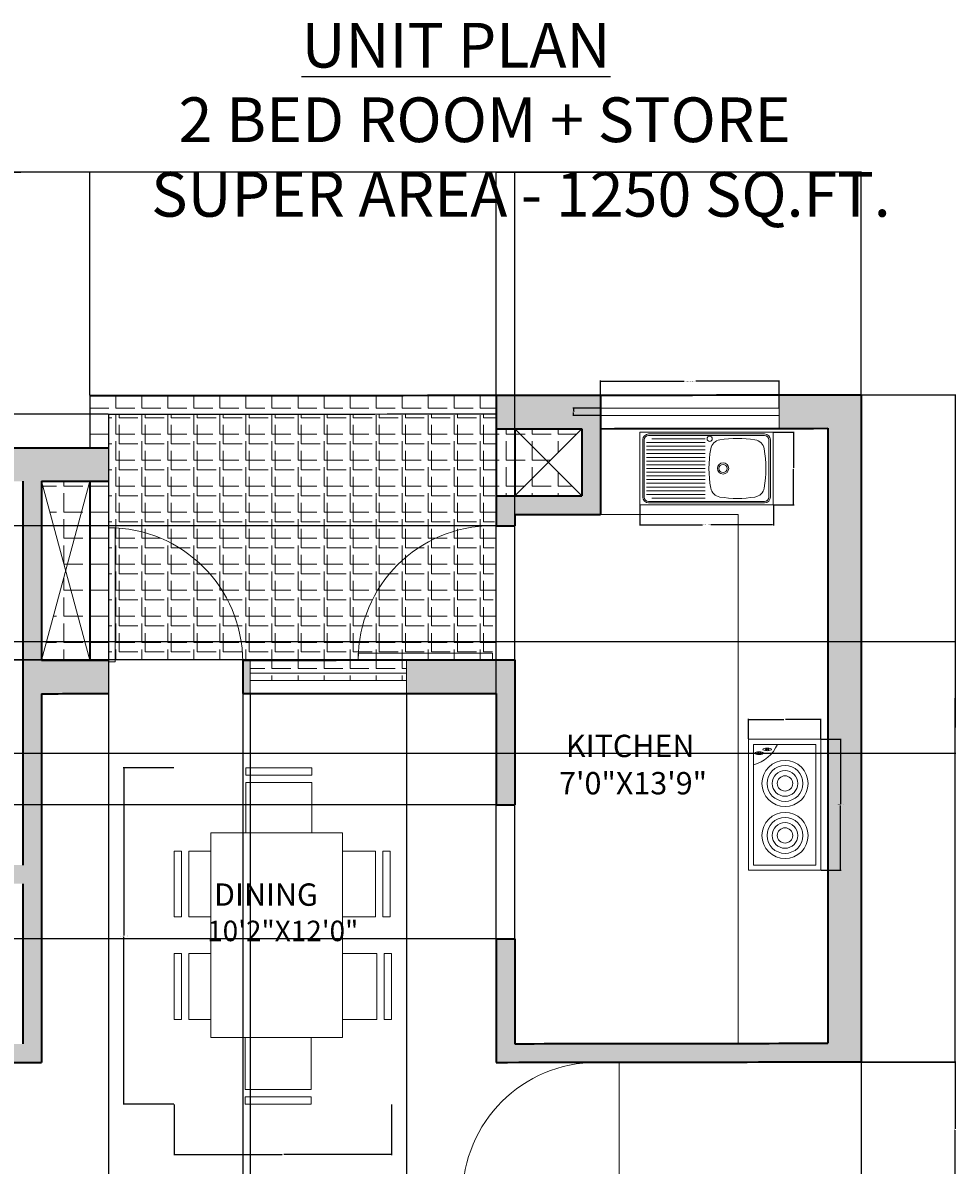
# Model space of a CAD drawing. Units: inches. Extents: x 1044 to 1567, y 918 to 1417.
# Tile 4 of 4: x 1316 to 1567, y 1110 to 1417. Entities that reach past the tile are written whole.
import ezdxf

# ---------------------------------------------------------------- set-up
doc = ezdxf.new("R2010")
doc.units = ezdxf.units.IN
for name, color, linetype, lineweight in [('A-ANNO-DIMS', 2, 'Continuous', 18), ('A-ANNO-TEXT', 7, 'Continuous', 25), ('A-AREA-IDEN', 7, 'Continuous', 18), ('A-EQPM', 8, 'Continuous', 18), ('A-FLOR', 7, 'Continuous', 13), ('A-FLOR-CASE', 8, 'Continuous', 18), ('A-FLOR-FIXT', 9, 'Continuous', 18), ('A-FLOR-OPEN', 8, 'Continuous', 13), ('A-FLOR-PATT', 9, 'Continuous', 13), ('A-FURN', 8, 'Continuous', 18), ('A-GLAZ', 4, 'Continuous', 13), ('A-WALL', 7, 'Continuous', 35), ('A-WALL-PATT', 252, 'Continuous', 13), ('A-WALL-PRPT', 7, 'Continuous', 25), ('door', 4, 'Continuous', 18)]:
    doc.layers.add(name, color=color, linetype=linetype, lineweight=lineweight)
doc.styles.get("Standard").update_dxf_attribs({"font": 'arial.ttf'})
doc.dimstyles.get("Standard").update_dxf_attribs({"dimtxt": 0.18, "dimasz": 0.18, "dimexe": 0.18, "dimexo": 0.0625, "dimgap": 0.09, "dimtad": 0, "dimtih": 1, "dimtoh": 1, "dimdec": 4, "dimzin": 0, "dimdsep": 46, "dimtxsty": 'Standard', "dimcen": 0.09, "dimadec": 0, "dimazin": 0, "dimtfac": 1, "dimtdec": 4, "dimtofl": 0, "dimtmove": 0, "dimatfit": 3, "dimfxl": 1, "dimtolj": 1, "dimtzin": 0, "dimarcsym": 0})

# ---------------------------------------------------------------- blocks, each defined once
blk = doc.blocks.new('*U5')
for p, q in [((-36, 0), (-36, 6)), ((0, 0), (0, 6))]:
    blk.add_line(p, q)
blk.add_lwpolyline([(0, 0), (0, -36), (-1.75, -36), (-1.75, 0)], close=True)
blk.add_arc((0, 0), 36, 180, 270)
blk = doc.blocks.new('*U2')
for p, q in [((0, 0), (0, -6)), ((36, 0), (36, -6))]:
    blk.add_line(p, q)
blk.add_lwpolyline([(0, 0), (0, 36), (1.75, 36), (1.75, 0)], close=True)
blk.add_arc((0, 0), 36, 0, 90)
blk = doc.blocks.new('A$C38705599')
for p, q in [((510, 282), (0, 282)), ((0, 282), (0, 0)), ((510, 0), (510, 282)), ((490, 262), (20, 262)), ((20, 262), (20, 20)), ((490, 20), (490, 262)), ((20, 20), (490, 20)), ((0, 0), (510, 0))]:
    blk.add_line(p, q)
for centre, radius in [((135.4, 139.5), 89.9), ((337.9, 139.5), 89.9), ((455.9, 243.8), 2.39), ((455.9, 235.1), 2.39), ((135.4, 139.5), 69.9), ((135.4, 139.5), 49.9), ((337.9, 139.5), 69.9), ((337.9, 139.5), 49.9), ((470.5, 213.1), 2.39), ((470.5, 204.3), 2.39), ((135.4, 139.5), 29.9), ((337.9, 139.5), 29.9)]:
    blk.add_circle(centre, radius)
blk.add_arc((552.1, 302.1), 147.4, 195.7794, 245.1074)
for centre in [(455.9, 239.9), (470.6, 209.1)]:
    blk.add_ellipse(centre, major_axis=(0, 17), ratio=0.307925)
blk = doc.blocks.new('A$C0C3933DC')
for p, q in [((0, 490), (0, 0)), ((900, 490), (0, 490)), ((59.5, 477.5), (450, 477.5)), ((59.5, 467.5), (450, 467.5)), ((840.5, 477.5), (450, 477.5)), ((840.5, 467.5), (450, 467.5)), ((900, 0), (900, 490)), ((19.5, 52.5), (19.5, 437.5)), ((29.5, 52.5), (29.5, 437.5)), ((441, 420), (45, 420)), ((441, 395), (45, 395)), ((441, 445), (80.7, 445)), ((870.5, 52.5), (870.5, 437.5)), ((880.5, 52.5), (880.5, 437.5)), ((441, 370), (45, 370)), ((441, 345), (45, 345)), ((441, 320), (45, 320)), ((441, 295), (45, 295)), ((441, 270), (45, 270)), ((441, 245), (45, 245)), ((441, 220), (45, 220)), ((441, 195), (45, 195)), ((441, 170), (45, 170)), ((441, 145), (45, 145)), ((441, 120), (45, 120)), ((441, 95), (45, 95)), ((0, 0), (900, 0)), ((441, 70), (45, 70)), ((450, 22.5), (59.5, 22.5)), ((450, 12.5), (59.5, 12.5)), ((441, 45), (80.7, 45)), ((450, 22.5), (840.5, 22.5)), ((450, 12.5), (840.5, 12.5))]:
    blk.add_line(p, q)
for centre, radius in [((471, 445), 17.5), ((561, 245), 38), ((561, 245), 27.5)]:
    blk.add_circle(centre, radius)
for centre, radius, start, end in [((59.5, 437.5), 40, 90, 180), ((59.5, 437.5), 30, 90, 180), ((840.5, 437.5), 40, 0, 90), ((840.5, 437.5), 30, 0, 90), ((551.5, 363.5), 75, 99.07872, 169.88522), ((658, -303), 750, 80.92128, 99.07872), ((764.5, 363.5), 75, 10.11478, 80.92128), ((1216, 245), 750, 169.88522, 190.11478), ((100, 245), 750, 349.88522, 10.11478), ((551.5, 126.5), 75, 190.11478, 260.92128), ((764.5, 126.5), 75, 279.07872, 349.88522), ((59.5, 52.5), 40, 180, 270), ((59.5, 52.5), 30, 180, 270), ((658, 793), 750, 260.92128, 279.07872), ((840.5, 52.5), 30, 270, 0), ((840.5, 52.5), 40, 270, 0)]:
    blk.add_arc(centre, radius, start, end)
blk = doc.blocks.new('A$C6F2E0C66')
for p, q in [((1.2673, 1.4847), (1.2673, 1.4347)), ((1.7173, 1.4847), (1.2673, 1.4847)), ((1.7173, 1.4347), (1.7173, 1.4847)), ((0.5675, 1.4758), (0.5675, 1.4258)), ((1.0175, 1.4758), (0.5675, 1.4758)), ((0.5675, 1.4258), (1.0175, 1.4258)), ((1.0175, 1.4258), (1.0175, 1.4758)), ((1.2673, 1.4347), (1.7173, 1.4347)), ((0.5675, 1.3758), (0.5675, 1.15)), ((1.0175, 1.3758), (0.5675, 1.3758)), ((1.0175, 1.15), (1.0175, 1.3758)), ((1.2673, 1.3847), (1.2673, 1.15)), ((1.7173, 1.3847), (1.2673, 1.3847)), ((1.7173, 1.15), (1.7173, 1.3847)), ((0.4423, 1.15), (0.4423, 0.25)), ((1.8423, 1.15), (0.4423, 1.15)), ((1.8423, 0.25), (1.8423, 1.15)), ((0, 0.9395), (0, 0.4895)), ((0.05, 0.9395), (0, 0.9395)), ((0.05, 0.4895), (0.05, 0.9395)), ((0.4423, 0.9395), (0.1, 0.9395)), ((0.1, 0.9395), (0.1, 0.4895)), ((2.197, 0.9346), (1.8423, 0.9346)), ((2.197, 0.4846), (2.197, 0.9346)), ((2.247, 0.9346), (2.247, 0.4846)), ((2.297, 0.9346), (2.247, 0.9346)), ((2.297, 0.4846), (2.297, 0.9346)), ((0, 0.4895), (0.05, 0.4895)), ((0.1, 0.4895), (0.4423, 0.4895)), ((1.8423, 0.4846), (2.197, 0.4846)), ((2.247, 0.4846), (2.297, 0.4846)), ((0.4423, 0.25), (1.8423, 0.25)), ((0.5675, 0.25), (0.5675, 0.1)), ((1.0175, 0.1), (1.0175, 0.25)), ((1.2678, 0.25), (1.2678, 0.1)), ((1.7178, 0.1), (1.7178, 0.25)), ((0.5675, 0.1), (1.0175, 0.1)), ((1.2678, 0.1), (1.7178, 0.1)), ((0.5675, 0.05), (0.5675, 0)), ((1.0175, 0.05), (0.5675, 0.05)), ((0.5675, 0), (1.0175, 0)), ((1.0175, 0), (1.0175, 0.05)), ((1.2678, 0.05), (1.2678, 0)), ((1.7178, 0.05), (1.2678, 0.05)), ((1.2678, 0), (1.7178, 0)), ((1.7178, 0), (1.7178, 0.05))]:
    blk.add_line(p, q)
blk = doc.blocks.new('GLAZ-PANEL-48IN')
for p, q in [((48, 2), (0, 2)), ((48, 0), (0, 0))]:
    blk.add_line(p, q)
blk = doc.blocks.new('*D20')
at = {"layer": 'A-ANNO-DIMS', "color": 0, "lineweight": -2, "transparency": 16777216}
for p, q in [((1471.18, 1313.26), (1471.18, 1320.57)), ((1471.36, 1320.39), (1493.62, 1320.39)), ((1519, 1320.39), (1496.74, 1320.39)), ((1519.18, 1313.26), (1519.18, 1320.57))]:
    blk.add_line(p, q, dxfattribs=at)
at = {"layer": 'A-ANNO-DIMS', "color": 0, "transparency": 16777216}
for points in [[(1471.36, 1320.42), (1471.36, 1320.36), (1471.18, 1320.39)], [(1519, 1320.42), (1519, 1320.36), (1519.18, 1320.39)]]:
    blk.add_solid(points, dxfattribs=at)
at = {"layer": 'Defpoints', "color": 0, "transparency": 16777216}
for p in [(1471.18, 1320.39), (1471.18, 1313.19), (1519.18, 1313.19)]:
    blk.add_point(p, dxfattribs=at)
at = {"layer": 'A-ANNO-DIMS', "color": 0, "transparency": 16777216, "insert": (1495.18, 1320.39), "char_height": 0.18, "attachment_point": 5}
blk.add_mtext('\\A1;GLAZING PANEL 48 TYP.', dxfattribs=at)
blk = doc.blocks.new('*D21')
at = {"layer": 'A-ANNO-DIMS', "color": 0, "lineweight": -2, "transparency": 16777216}
for p, q in [((1471.11, 1313.19), (1463.8, 1313.19)), ((1463.98, 1313.01), (1463.98, 1312.37)), ((1463.98, 1311.37), (1463.98, 1312.01)), ((1471.11, 1311.19), (1463.8, 1311.19))]:
    blk.add_line(p, q, dxfattribs=at)
at = {"layer": 'A-ANNO-DIMS', "color": 0, "transparency": 16777216}
for points in [[(1463.95, 1313.01), (1464.01, 1313.01), (1463.98, 1313.19)], [(1463.95, 1311.37), (1464.01, 1311.37), (1463.98, 1311.19)]]:
    blk.add_solid(points, dxfattribs=at)
at = {"layer": 'Defpoints', "color": 0, "transparency": 16777216}
for p in [(1471.18, 1313.19), (1463.98, 1311.19), (1471.18, 1311.19)]:
    blk.add_point(p, dxfattribs=at)
at = {"layer": 'A-ANNO-DIMS', "color": 0, "transparency": 16777216, "insert": (1463.98, 1312.19), "char_height": 0.18, "attachment_point": 5}
blk.add_mtext('\\A1;2 TYP.', dxfattribs=at)
blk = doc.blocks.new('*D24')
at = {"layer": 'A-ANNO-DIMS', "color": 0, "lineweight": -2, "transparency": 16777216}
for p, q in [((1530.39, 1224.32), (1535.78, 1224.32)), ((1535.6, 1224.14), (1535.6, 1206.93)), ((1535.6, 1189.36), (1535.6, 1206.57)), ((1530.39, 1189.18), (1535.78, 1189.18))]:
    blk.add_line(p, q, dxfattribs=at)
at = {"layer": 'A-ANNO-DIMS', "color": 0, "transparency": 16777216}
for points in [[(1535.57, 1224.14), (1535.63, 1224.14), (1535.6, 1224.32)], [(1535.57, 1189.36), (1535.63, 1189.36), (1535.6, 1189.18)]]:
    blk.add_solid(points, dxfattribs=at)
at = {"layer": 'Defpoints', "color": 0, "transparency": 16777216}
for p in [(1530.33, 1224.32), (1535.6, 1224.32), (1530.33, 1189.18)]:
    blk.add_point(p, dxfattribs=at)
at = {"layer": 'A-ANNO-DIMS', "color": 0, "transparency": 16777216, "insert": (1535.6, 1206.75), "char_height": 0.18, "attachment_point": 5}
blk.add_mtext('\\A1;COOKTOP 35', dxfattribs=at)
blk = doc.blocks.new('*D25')
at = {"layer": 'A-ANNO-DIMS', "color": 0, "lineweight": -2, "transparency": 16777216}
for p, q in [((1510.89, 1224.39), (1510.89, 1229.78)), ((1511.07, 1229.6), (1520.4, 1229.6)), ((1530.15, 1229.6), (1520.82, 1229.6)), ((1530.33, 1224.39), (1530.33, 1229.78))]:
    blk.add_line(p, q, dxfattribs=at)
at = {"layer": 'A-ANNO-DIMS', "color": 0, "transparency": 16777216}
for points in [[(1511.07, 1229.63), (1511.07, 1229.57), (1510.89, 1229.6)], [(1530.15, 1229.63), (1530.15, 1229.57), (1530.33, 1229.6)]]:
    blk.add_solid(points, dxfattribs=at)
at = {"layer": 'Defpoints', "color": 0, "transparency": 16777216}
for p in [(1510.89, 1229.6), (1510.89, 1224.32), (1530.33, 1224.32)]:
    blk.add_point(p, dxfattribs=at)
at = {"layer": 'A-ANNO-DIMS', "color": 0, "transparency": 16777216, "insert": (1520.61, 1229.6), "char_height": 0.18, "attachment_point": 5}
blk.add_mtext('\\A1;19', dxfattribs=at)
blk = doc.blocks.new('*D26')
at = {"layer": 'A-ANNO-DIMS', "color": 0, "lineweight": -2, "transparency": 16777216}
for p, q in [((1481.75, 1287.17), (1481.75, 1281.68)), ((1517.58, 1287.17), (1517.58, 1281.68)), ((1481.93, 1281.86), (1498.54, 1281.86)), ((1517.4, 1281.86), (1500.8, 1281.86))]:
    blk.add_line(p, q, dxfattribs=at)
at = {"layer": 'A-ANNO-DIMS', "color": 0, "transparency": 16777216}
for points in [[(1481.93, 1281.89), (1481.93, 1281.83), (1481.75, 1281.86)], [(1517.4, 1281.89), (1517.4, 1281.83), (1517.58, 1281.86)]]:
    blk.add_solid(points, dxfattribs=at)
at = {"layer": 'Defpoints', "color": 0, "transparency": 16777216}
for p in [(1481.75, 1287.23), (1517.58, 1287.23), (1517.58, 1281.86)]:
    blk.add_point(p, dxfattribs=at)
at = {"layer": 'A-ANNO-DIMS', "color": 0, "transparency": 16777216, "insert": (1499.67, 1281.86), "char_height": 0.18, "attachment_point": 5}
blk.add_mtext('\\A1;KITCHEN SINK 36', dxfattribs=at)
blk = doc.blocks.new('*D27')
at = {"layer": 'A-ANNO-DIMS', "color": 0, "lineweight": -2, "transparency": 16777216}
for p, q in [((1517.64, 1306.73), (1523.13, 1306.73)), ((1522.95, 1306.55), (1522.95, 1297.16)), ((1522.95, 1287.41), (1522.95, 1296.8)), ((1517.64, 1287.23), (1523.13, 1287.23))]:
    blk.add_line(p, q, dxfattribs=at)
at = {"layer": 'A-ANNO-DIMS', "color": 0, "transparency": 16777216}
for points in [[(1522.92, 1306.55), (1522.98, 1306.55), (1522.95, 1306.73)], [(1522.92, 1287.41), (1522.98, 1287.41), (1522.95, 1287.23)]]:
    blk.add_solid(points, dxfattribs=at)
at = {"layer": 'Defpoints', "color": 0, "transparency": 16777216}
for p in [(1517.58, 1306.73), (1522.95, 1306.73), (1517.58, 1287.23)]:
    blk.add_point(p, dxfattribs=at)
at = {"layer": 'A-ANNO-DIMS', "color": 0, "transparency": 16777216, "insert": (1522.95, 1296.98), "char_height": 0.18, "attachment_point": 5}
blk.add_mtext('\\A1;20', dxfattribs=at)
blk = doc.blocks.new('*D28')
at = {"layer": 'A-ANNO-DIMS', "color": 0, "lineweight": -2, "transparency": 16777216}
for p, q in [((1356.74, 1216.62), (1343.09, 1216.62)), ((1343.27, 1216.44), (1343.27, 1171.69)), ((1343.27, 1126.57), (1343.27, 1171.32)), ((1356.74, 1126.39), (1343.09, 1126.39))]:
    blk.add_line(p, q, dxfattribs=at)
at = {"layer": 'A-ANNO-DIMS', "color": 0, "transparency": 16777216}
for points in [[(1343.24, 1216.44), (1343.3, 1216.44), (1343.27, 1216.62)], [(1343.24, 1126.57), (1343.3, 1126.57), (1343.27, 1126.39)]]:
    blk.add_solid(points, dxfattribs=at)
at = {"layer": 'Defpoints', "color": 0, "transparency": 16777216}
for p in [(1356.8, 1216.62), (1343.27, 1126.39), (1356.8, 1126.39)]:
    blk.add_point(p, dxfattribs=at)
at = {"layer": 'A-ANNO-DIMS', "color": 0, "transparency": 16777216, "insert": (1343.27, 1171.51), "char_height": 0.18, "attachment_point": 5}
blk.add_mtext('\\A1;DINING GROUP 90', dxfattribs=at)
blk = doc.blocks.new('*D29')
at = {"layer": 'A-ANNO-DIMS', "color": 0, "lineweight": -2, "transparency": 16777216}
for p, q in [((1356.8, 1126.33), (1356.8, 1112.68)), ((1415.12, 1126.33), (1415.12, 1112.68)), ((1356.98, 1112.86), (1385.74, 1112.86)), ((1414.94, 1112.86), (1386.18, 1112.86))]:
    blk.add_line(p, q, dxfattribs=at)
at = {"layer": 'A-ANNO-DIMS', "color": 0, "transparency": 16777216}
for points in [[(1356.98, 1112.89), (1356.98, 1112.83), (1356.8, 1112.86)], [(1414.94, 1112.89), (1414.94, 1112.83), (1415.12, 1112.86)]]:
    blk.add_solid(points, dxfattribs=at)
at = {"layer": 'Defpoints', "color": 0, "transparency": 16777216}
for p in [(1356.8, 1126.39), (1415.12, 1126.39), (1415.12, 1112.86)]:
    blk.add_point(p, dxfattribs=at)
at = {"layer": 'A-ANNO-DIMS', "color": 0, "transparency": 16777216, "insert": (1385.96, 1112.86), "char_height": 0.18, "attachment_point": 5}
blk.add_mtext('\\A1;58', dxfattribs=at)
blk = doc.blocks.new('*D30')
at = {"layer": 'A-ANNO-DIMS', "color": 0, "lineweight": -2, "transparency": 16777216}
for p, q in [((1069.18, 1283.83), (1069.18, 1376.67)), ((1069.36, 1376.49), (1304.89, 1376.49)), ((1541, 1376.49), (1305.47, 1376.49)), ((1541.18, 1316.83), (1541.18, 1376.67))]:
    blk.add_line(p, q, dxfattribs=at)
at = {"layer": 'A-ANNO-DIMS', "color": 0, "transparency": 16777216}
for points in [[(1069.36, 1376.52), (1069.36, 1376.46), (1069.18, 1376.49)], [(1541, 1376.52), (1541, 1376.46), (1541.18, 1376.49)]]:
    blk.add_solid(points, dxfattribs=at)
at = {"layer": 'Defpoints', "color": 0, "transparency": 16777216}
for p in [(1541.18, 1376.49), (1541.18, 1316.77), (1069.18, 1283.77)]:
    blk.add_point(p, dxfattribs=at)
at = {"layer": 'A-ANNO-DIMS', "color": 0, "transparency": 16777216, "insert": (1305.18, 1376.49), "char_height": 0.18, "attachment_point": 5}
blk.add_mtext('\\A1;472', dxfattribs=at)
blk = doc.blocks.new('*D35')
at = {"layer": 'A-ANNO-DIMS', "color": 0, "lineweight": -2, "transparency": 16777216}
for p, q in [((1541.18, 1137.7), (1541.18, 918.44)), ((1452.18, 945.57), (1452.18, 918.44)), ((1452.36, 918.62), (1496.46, 918.62)), ((1541, 918.62), (1496.9, 918.62))]:
    blk.add_line(p, q, dxfattribs=at)
at = {"layer": 'A-ANNO-DIMS', "color": 0, "transparency": 16777216}
for points in [[(1452.36, 918.65), (1452.36, 918.59), (1452.18, 918.62)], [(1541, 918.65), (1541, 918.59), (1541.18, 918.62)]]:
    blk.add_solid(points, dxfattribs=at)
at = {"layer": 'Defpoints', "color": 0, "transparency": 16777216}
for p in [(1541.18, 1137.77), (1452.18, 945.63), (1541.18, 918.62)]:
    blk.add_point(p, dxfattribs=at)
at = {"layer": 'A-ANNO-DIMS', "color": 0, "transparency": 16777216, "insert": (1496.68, 918.62), "char_height": 0.18, "attachment_point": 5}
blk.add_mtext('\\A1;89', dxfattribs=at)
blk = doc.blocks.new('*D38')
at = {"layer": 'A-ANNO-DIMS', "color": 0, "lineweight": -2, "transparency": 16777216}
for p, q in [((1476.24, 1137.66), (1566.52, 1137.66)), ((1566.34, 1137.48), (1566.34, 1119.83)), ((1566.34, 1101.82), (1566.34, 1119.47)), ((1476.24, 1101.64), (1566.52, 1101.64))]:
    blk.add_line(p, q, dxfattribs=at)
at = {"layer": 'A-ANNO-DIMS', "color": 0, "transparency": 16777216}
for points in [[(1566.31, 1137.48), (1566.37, 1137.48), (1566.34, 1137.66)], [(1566.31, 1101.82), (1566.37, 1101.82), (1566.34, 1101.64)]]:
    blk.add_solid(points, dxfattribs=at)
at = {"layer": 'Defpoints', "color": 0, "transparency": 16777216}
for p in [(1476.18, 1137.66), (1566.34, 1137.66), (1476.18, 1101.64)]:
    blk.add_point(p, dxfattribs=at)
at = {"layer": 'A-ANNO-DIMS', "color": 0, "transparency": 16777216, "insert": (1566.34, 1119.65), "char_height": 0.18, "attachment_point": 5}
blk.add_mtext('\\A1;36.03', dxfattribs=at)
blk = doc.blocks.new('*D39')
at = {"layer": 'A-ANNO-DIMS', "color": 0, "lineweight": -2, "transparency": 16777216}
for p, q in [((1541.24, 1316.77), (1566.52, 1316.77)), ((1566.34, 1316.59), (1566.34, 1227.45)), ((1566.34, 1137.95), (1566.34, 1227.09)), ((1541.24, 1137.77), (1566.52, 1137.77))]:
    blk.add_line(p, q, dxfattribs=at)
at = {"layer": 'A-ANNO-DIMS', "color": 0, "transparency": 16777216}
for points in [[(1566.31, 1316.59), (1566.37, 1316.59), (1566.34, 1316.77)], [(1566.31, 1137.95), (1566.37, 1137.95), (1566.34, 1137.77)]]:
    blk.add_solid(points, dxfattribs=at)
at = {"layer": 'Defpoints', "color": 0, "transparency": 16777216}
for p in [(1541.18, 1316.77), (1566.34, 1316.77), (1541.18, 1137.77)]:
    blk.add_point(p, dxfattribs=at)
at = {"layer": 'A-ANNO-DIMS', "color": 0, "transparency": 16777216, "insert": (1566.34, 1227.27), "char_height": 0.18, "attachment_point": 5}
blk.add_mtext('\\A1;179', dxfattribs=at)
blk = doc.blocks.new('*D44')
at = {"layer": 'A-ANNO-DIMS', "color": 0, "lineweight": -2, "transparency": 16777216}
for p, q in [((1297.68, 1302.62), (1297.68, 1376.67)), ((1297.86, 1376.49), (1315.6, 1376.49)), ((1334, 1376.49), (1316.25, 1376.49)), ((1334.18, 1316.62), (1334.18, 1376.67))]:
    blk.add_line(p, q, dxfattribs=at)
at = {"layer": 'A-ANNO-DIMS', "color": 0, "transparency": 16777216}
for points in [[(1297.86, 1376.52), (1297.86, 1376.46), (1297.68, 1376.49)], [(1334, 1376.52), (1334, 1376.46), (1334.18, 1376.49)]]:
    blk.add_solid(points, dxfattribs=at)
at = {"layer": 'Defpoints', "color": 0, "transparency": 16777216}
for p in [(1334.18, 1376.49), (1334.18, 1316.55), (1297.68, 1302.55)]:
    blk.add_point(p, dxfattribs=at)
at = {"layer": 'A-ANNO-DIMS', "color": 0, "transparency": 16777216, "insert": (1315.93, 1376.49), "char_height": 0.18, "attachment_point": 5}
blk.add_mtext('\\A1;36.5', dxfattribs=at)
blk = doc.blocks.new('*D45')
at = {"layer": 'A-ANNO-DIMS', "color": 0, "lineweight": -2, "transparency": 16777216}
for p, q in [((1443.18, 1316.69), (1443.18, 1376.67)), ((1443.36, 1376.49), (1491.96, 1376.49)), ((1541, 1376.49), (1492.4, 1376.49)), ((1541.18, 1316.83), (1541.18, 1376.67))]:
    blk.add_line(p, q, dxfattribs=at)
at = {"layer": 'A-ANNO-DIMS', "color": 0, "transparency": 16777216}
for points in [[(1443.36, 1376.52), (1443.36, 1376.46), (1443.18, 1376.49)], [(1541, 1376.52), (1541, 1376.46), (1541.18, 1376.49)]]:
    blk.add_solid(points, dxfattribs=at)
at = {"layer": 'Defpoints', "color": 0, "transparency": 16777216}
for p in [(1541.18, 1376.49), (1443.18, 1316.63), (1541.18, 1316.77)]:
    blk.add_point(p, dxfattribs=at)
at = {"layer": 'A-ANNO-DIMS', "color": 0, "transparency": 16777216, "insert": (1492.18, 1376.49), "char_height": 0.18, "attachment_point": 5}
blk.add_mtext('\\A1;98', dxfattribs=at)
blk = doc.blocks.new('*D51')
at = {"layer": 'A-ANNO-DIMS', "color": 0, "lineweight": -2, "transparency": 16777216}
for p, q in [((1443.11, 1206.74), (1043.83, 1206.74)), ((1044.01, 1206.56), (1044.01, 1188.92)), ((1044.01, 1170.92), (1044.01, 1188.56)), ((1443.11, 1170.74), (1043.83, 1170.74))]:
    blk.add_line(p, q, dxfattribs=at)
at = {"layer": 'A-ANNO-DIMS', "color": 0, "transparency": 16777216}
for points in [[(1043.98, 1206.56), (1044.04, 1206.56), (1044.01, 1206.74)], [(1043.98, 1170.92), (1044.04, 1170.92), (1044.01, 1170.74)]]:
    blk.add_solid(points, dxfattribs=at)
at = {"layer": 'Defpoints', "color": 0, "transparency": 16777216}
for p in [(1044.01, 1206.74), (1443.18, 1206.74), (1443.18, 1170.74)]:
    blk.add_point(p, dxfattribs=at)
at = {"layer": 'A-ANNO-DIMS', "color": 0, "transparency": 16777216, "insert": (1044.01, 1188.74), "char_height": 0.18, "attachment_point": 5}
blk.add_mtext('\\A1;36', dxfattribs=at)
blk = doc.blocks.new('*D52')
at = {"layer": 'A-ANNO-DIMS', "color": 0, "lineweight": -2, "transparency": 16777216}
for p, q in [((1443.18, 1170.8), (1443.18, 1376.67)), ((1443.36, 1376.49), (1445.53, 1376.49)), ((1448, 1376.49), (1445.83, 1376.49)), ((1448.18, 1170.8), (1448.18, 1376.67))]:
    blk.add_line(p, q, dxfattribs=at)
at = {"layer": 'A-ANNO-DIMS', "color": 0, "transparency": 16777216}
for points in [[(1443.36, 1376.52), (1443.36, 1376.46), (1443.18, 1376.49)], [(1448, 1376.52), (1448, 1376.46), (1448.18, 1376.49)]]:
    blk.add_solid(points, dxfattribs=at)
at = {"layer": 'Defpoints', "color": 0, "transparency": 16777216}
for p in [(1448.18, 1376.49), (1443.18, 1170.74), (1448.18, 1170.74)]:
    blk.add_point(p, dxfattribs=at)
at = {"layer": 'A-ANNO-DIMS', "color": 0, "transparency": 16777216, "insert": (1445.68, 1376.49), "char_height": 0.18, "attachment_point": 5}
blk.add_mtext('\\A1;5', dxfattribs=at)
blk = doc.blocks.new('*D53')
at = {"layer": 'A-ANNO-DIMS', "color": 0, "lineweight": -2, "transparency": 16777216}
for p, q in [((1255.24, 1250.56), (1566.52, 1250.56)), ((1566.34, 1250.38), (1566.34, 1235.74)), ((1566.34, 1220.74), (1566.34, 1235.38)), ((1255.24, 1220.56), (1566.52, 1220.56))]:
    blk.add_line(p, q, dxfattribs=at)
at = {"layer": 'A-ANNO-DIMS', "color": 0, "transparency": 16777216}
for points in [[(1566.31, 1250.38), (1566.37, 1250.38), (1566.34, 1250.56)], [(1566.31, 1220.74), (1566.37, 1220.74), (1566.34, 1220.56)]]:
    blk.add_solid(points, dxfattribs=at)
at = {"layer": 'Defpoints', "color": 0, "transparency": 16777216}
for p in [(1255.18, 1250.56), (1566.34, 1250.56), (1255.18, 1220.56)]:
    blk.add_point(p, dxfattribs=at)
at = {"layer": 'A-ANNO-DIMS', "color": 0, "transparency": 16777216, "insert": (1566.34, 1235.56), "char_height": 0.18, "attachment_point": 5}
blk.add_mtext('\\A1;30', dxfattribs=at)
blk = doc.blocks.new('*D58')
at = {"layer": 'A-ANNO-DIMS', "color": 0, "lineweight": -2, "transparency": 16777216}
for p, q in [((1339.18, 1236.49), (1339.18, 918.44)), ((1375.18, 1236.49), (1375.18, 918.44)), ((1339.36, 918.62), (1356.96, 918.62)), ((1375, 918.62), (1357.4, 918.62))]:
    blk.add_line(p, q, dxfattribs=at)
at = {"layer": 'A-ANNO-DIMS', "color": 0, "transparency": 16777216}
for points in [[(1339.36, 918.65), (1339.36, 918.59), (1339.18, 918.62)], [(1375, 918.65), (1375, 918.59), (1375.18, 918.62)]]:
    blk.add_solid(points, dxfattribs=at)
at = {"layer": 'Defpoints', "color": 0, "transparency": 16777216}
for p in [(1339.18, 1236.56), (1375.18, 1236.56), (1375.18, 918.62)]:
    blk.add_point(p, dxfattribs=at)
at = {"layer": 'A-ANNO-DIMS', "color": 0, "transparency": 16777216, "insert": (1357.18, 918.62), "char_height": 0.18, "attachment_point": 5}
blk.add_mtext('\\A1;36', dxfattribs=at)
blk = doc.blocks.new('*D59')
at = {"layer": 'A-ANNO-DIMS', "color": 0, "lineweight": -2, "transparency": 16777216}
for p, q in [((1377.18, 1236.49), (1377.18, 918.44)), ((1419.18, 1236.49), (1419.18, 918.44)), ((1377.36, 918.62), (1397.96, 918.62)), ((1419, 918.62), (1398.4, 918.62))]:
    blk.add_line(p, q, dxfattribs=at)
at = {"layer": 'A-ANNO-DIMS', "color": 0, "transparency": 16777216}
for points in [[(1377.36, 918.65), (1377.36, 918.59), (1377.18, 918.62)], [(1419, 918.65), (1419, 918.59), (1419.18, 918.62)]]:
    blk.add_solid(points, dxfattribs=at)
at = {"layer": 'Defpoints', "color": 0, "transparency": 16777216}
for p in [(1377.18, 1236.56), (1419.18, 1236.56), (1419.18, 918.62)]:
    blk.add_point(p, dxfattribs=at)
at = {"layer": 'A-ANNO-DIMS', "color": 0, "transparency": 16777216, "insert": (1398.18, 918.62), "char_height": 0.18, "attachment_point": 5}
blk.add_mtext('\\A1;42', dxfattribs=at)
blk = doc.blocks.new('*D60')
at = {"layer": 'A-ANNO-DIMS', "color": 0, "lineweight": -2, "transparency": 16777216}
for p, q in [((1443.11, 1281.62), (1043.83, 1281.62)), ((1044.01, 1281.44), (1044.01, 1263.79)), ((1044.01, 1245.78), (1044.01, 1263.43)), ((1443.15, 1245.6), (1043.83, 1245.6))]:
    blk.add_line(p, q, dxfattribs=at)
at = {"layer": 'A-ANNO-DIMS', "color": 0, "transparency": 16777216}
for points in [[(1043.98, 1281.44), (1044.04, 1281.44), (1044.01, 1281.62)], [(1043.98, 1245.78), (1044.04, 1245.78), (1044.01, 1245.6)]]:
    blk.add_solid(points, dxfattribs=at)
at = {"layer": 'Defpoints', "color": 0, "transparency": 16777216}
for p in [(1044.01, 1281.62), (1443.18, 1281.62), (1443.22, 1245.6)]:
    blk.add_point(p, dxfattribs=at)
at = {"layer": 'A-ANNO-DIMS', "color": 0, "transparency": 16777216, "insert": (1044.01, 1263.61), "char_height": 0.18, "attachment_point": 5}
blk.add_mtext('\\A1;36.03', dxfattribs=at)
blk = doc.blocks.new('*D61')
at = {"layer": 'A-ANNO-DIMS', "color": 0, "lineweight": -2, "transparency": 16777216}
for p, q in [((1339.11, 1311.56), (1043.83, 1311.56)), ((1044.01, 1311.38), (1044.01, 1278.74)), ((1044.01, 1245.74), (1044.01, 1278.37)), ((1339.11, 1245.56), (1043.83, 1245.56))]:
    blk.add_line(p, q, dxfattribs=at)
at = {"layer": 'A-ANNO-DIMS', "color": 0, "transparency": 16777216}
for points in [[(1043.98, 1311.38), (1044.04, 1311.38), (1044.01, 1311.56)], [(1043.98, 1245.74), (1044.04, 1245.74), (1044.01, 1245.56)]]:
    blk.add_solid(points, dxfattribs=at)
at = {"layer": 'Defpoints', "color": 0, "transparency": 16777216}
for p in [(1044.01, 1311.56), (1339.18, 1311.56), (1339.18, 1245.56)]:
    blk.add_point(p, dxfattribs=at)
at = {"layer": 'A-ANNO-DIMS', "color": 0, "transparency": 16777216, "insert": (1044.01, 1278.56), "char_height": 0.18, "attachment_point": 5}
blk.add_mtext('\\A1;66', dxfattribs=at)

msp = doc.modelspace()

# ---------------------------------------------------------------- hatches: boundary and pattern name
at = {"layer": 'A-FLOR-PATT'}
h = msp.add_hatch(dxfattribs=at)
h.set_pattern_fill('ANGLE', color=256)
h.set_pattern_definition([(0, (0, 0), (0, 6.985), [5.08, -1.905]), (90, (0, 0), (-6.985, 4e-16), [5.08, -1.905])])
h.paths.add_polyline_path([(1142.177, 1283.654, -0.0000039), (1140.177, 1283.657), (1140.177, 1278.134), (1092.177, 1278.134), (1092.177, 1283.727, -0.0000097), (1087.177, 1283.735), (1087.177, 1337.654), (1183.177, 1337.654), (1183.177, 1302.563), (1178.177, 1302.563), (1178.177, 1283.654)])
h.paths.add_polyline_path([(1321.177, 1245.553), (1327.676, 1269.552), (1321.174, 1293.553, 0.0000348), (1339.177, 1293.556), (1339.177, 1302.556, -0.0000097), (1334.177, 1302.555), (1334.177, 1316.555, 0.0002109), (1443.177, 1316.625), (1443.177, 1307.625, 0.0000445), (1466.198, 1307.652), (1457.182, 1298.636), (1466.177, 1289.652, -0.0000445), (1443.177, 1289.625), (1443.177, 1281.625), (1443.215, 1245.625, -0.0000465), (1419.177, 1245.602), (1419.177, 1240.063), (1377.177, 1240.063), (1377.177, 1245.572, -0.0000039), (1375.177, 1245.571), (1339.177, 1245.556, -0.0000348)])
h = msp.add_hatch(dxfattribs=at)
h.set_pattern_fill('ANGLE', color=256)
h.set_pattern_definition([(0, (252.329, -30.523), (0, 6.985), [5.08, -1.905]), (90, (252.329, -30.523), (-6.985, 4e-16), [5.08, -1.905])])
edge = h.paths.add_edge_path()
edge.add_line((1443.177, 1311.625), (1339.177, 1311.556))
edge.add_line((1339.177, 1311.556), (1339.177, 1245.556))
edge.add_arc((1391.878, -412.698), 1659.092, 88.262695, 91.820313, ccw=False)
edge.add_line((1442.177, 1245.631), (1443.177, 1311.625))
at = {"layer": 'A-WALL-PATT'}
h = msp.add_hatch(color=256, dxfattribs=at)
h.dxf.hatch_style = 1
h.paths.add_polyline_path([(1541.177, 1316.767, -0.0000426), (1519.177, 1316.729), (1519.177, 1307.729, 0.0000252), (1532.177, 1307.751), (1532.177, 1142.751, -0.0001623), (1448.177, 1142.631), (1448.177, 1170.739), (1443.177, 1170.739), (1443.177, 1137.625, 0.0001894), (1541.177, 1137.767)])
h = msp.add_hatch(color=256, dxfattribs=at)
h.dxf.hatch_style = 1
h.paths.add_polyline_path([(1471.177, 1316.658, -0.0000542), (1443.177, 1316.625), (1443.177, 1307.625, 0.0000445), (1466.198, 1307.652), (1466.177, 1307.631), (1466.177, 1289.652, -0.0000445), (1443.177, 1289.625), (1443.177, 1281.625, 0.0000089), (1448.177, 1281.63), (1448.177, 1284.631, 0.0000445), (1471.177, 1284.658)])
h = msp.add_hatch(color=256, dxfattribs=at)
h.dxf.hatch_style = 1
h.paths.add_polyline_path([(1273.677, 1302.555, -0.0000455), (1250.177, 1302.563), (1178.177, 1302.563), (1178.177, 1274.614, 0.0000213), (1189.177, 1274.604), (1189.177, 1279.604, -0.0000116), (1183.177, 1279.609), (1183.177, 1297.563), (1250.177, 1297.563), (1250.177, 1250.563, 0.0000097), (1255.177, 1250.561), (1255.177, 1293.561, 0.0000358), (1273.677, 1293.555)])
h.paths.add_polyline_path([(1339.177, 1302.556, -0.0000348), (1321.176, 1302.553, -0.0000455), (1297.677, 1302.552), (1297.677, 1293.552, 0.0000358), (1316.177, 1293.552), (1316.177, 1190.552, -0.0001179), (1255.177, 1190.561), (1255.177, 1220.561, -0.0000097), (1250.177, 1220.563), (1250.177, 1137.563, 0.0000097), (1255.177, 1137.561), (1255.177, 1185.561, 0.0001179), (1316.177, 1185.552), (1316.177, 1142.552, -0.0000483), (1291.177, 1142.552), (1291.177, 1137.552, 0.000058), (1321.177, 1137.553), (1321.177, 1236.553, 0.0000348), (1339.177, 1236.556), (1339.177, 1245.556, -0.0000348), (1321.177, 1245.553), (1321.177, 1293.544), (1321.174, 1293.553, 0.0000348), (1339.177, 1293.556)])
h = msp.add_hatch(color=256, dxfattribs=at)
h.dxf.hatch_style = 1
h.paths.add_polyline_path([(1448.177, 1245.631, -0.0000561), (1419.177, 1245.602), (1419.177, 1236.602, 0.0000464), (1443.177, 1236.625), (1443.177, 1206.739), (1448.177, 1206.739)])
h.paths.add_polyline_path([(1377.177, 1245.572, -0.0000039), (1375.177, 1245.571), (1375.177, 1236.571, 0.0000039), (1377.177, 1236.572)])

# ---------------------------------------------------------------- linework, layer by layer
at = {"layer": 'A-FLOR'}
for p, q in [((1448.177, 1245.631), (1448.13, 1289.631)), ((1443.215, 1245.598), (1339.177, 1245.556)), ((1476.177, 1092.635), (1476.177, 1137.665))]:
    msp.add_line(p, q, dxfattribs=at)
at = {"layer": 'A-FLOR-CASE'}
for p, q in [((1471.177, 1284.658), (1508.177, 1284.658)), ((1508.177, 1284.658), (1508.177, 1142.751))]:
    msp.add_line(p, q, dxfattribs=at)
at = {"layer": 'A-FLOR-OPEN'}
for p, q in [((1448.177, 1289.631), (1466.177, 1307.631)), ((1466.177, 1289.652), (1448.177, 1307.631)), ((1334.177, 1245.555), (1321.174, 1293.553)), ((1334.177, 1293.555), (1321.177, 1245.553))]:
    msp.add_line(p, q, dxfattribs=at)
at = {"layer": 'A-GLAZ'}
for p, q in [((1519.177, 1316.658), (1519.177, 1307.729)), ((1377.177, 1245.571), (1377.177, 1236.556)), ((1419.177, 1245.571), (1419.177, 1236.556)), ((1419.177, 1242.063), (1377.177, 1242.063)), ((1419.177, 1240.063), (1377.177, 1240.063))]:
    msp.add_line(p, q, dxfattribs=at)
at = {"layer": 'A-WALL'}
for p, q in [((1443.177, 1316.625), (1443.177, 1281.625)), ((1471.177, 1316.658), (1471.177, 1284.658)), ((1541.177, 1316.767), (1541.177, 1137.767)), ((1448.177, 1307.631), (1448.177, 1289.631)), ((1466.177, 1307.652), (1466.177, 1289.652)), ((1532.177, 1307.751), (1532.177, 1142.751)), ((1316.177, 1293.552), (1316.177, 1190.552)), ((1321.177, 1293.553), (1321.177, 1245.553)), ((1334.177, 1293.555), (1334.177, 1245.555)), ((1448.177, 1284.631), (1448.177, 1281.63)), ((1375.177, 1245.571), (1375.177, 1236.556)), ((1448.177, 1245.631), (1448.177, 1206.739)), ((1321.177, 1236.553), (1321.177, 1137.553)), ((1443.177, 1236.625), (1443.177, 1206.739)), ((1443.177, 1206.739), (1448.177, 1206.739)), ((1316.177, 1185.552), (1316.177, 1142.552)), ((1443.177, 1170.739), (1448.177, 1170.739)), ((1443.177, 1170.739), (1443.177, 1137.625)), ((1448.177, 1170.739), (1448.177, 1142.631))]:
    msp.add_line(p, q, dxfattribs=at)
for centre, radius, start, end in [((1305.177, 130508.416), 129191.864, 270.01286132, 270.10466457), ((1305.177, 130508.416), 129196.864, 270.10466052, 270.10466457), ((1305.177, 130508.416), 129200.864, 270.06119788, 270.07139753), ((1305.177, 130508.416), 129200.864, 270.07361485, 270.10066611), ((1305.177, 130508.416), 129205.864, 269.97561049, 270.00709513), ((1305.174, 130539.416), 129236.864, 270.00709343, 270.01507458), ((1305.174, 130539.416), 129245.864, 270.00709293, 270.01507353), ((1305.177, 130508.416), 129218.864, 270.06118936, 270.07138759), ((1305.177, 130508.416), 129223.864, 270.06340391, 270.07360175), ((1297.237, 142167.97), 140886.421, 270.05935085, 270.06138426), ((1305.174, 130539.416), 129293.864, 270.00709134, 270.01506793), ((1305.174, 130539.416), 129293.864, 270.03102111, 270.06337062), ((1305.174, 130539.416), 129302.864, 270.00709085, 270.01506688), ((1305.174, 130539.416), 129302.864, 270.03101895, 270.06115065), ((1305.177, 130508.416), 129365.864, 270.06333431, 270.10053772), ((1305.177, 130508.416), 129370.864, 269.99379968, 270.00708608), ((1305.177, 130508.416), 129370.864, 270.06111746, 270.10451976)]:
    msp.add_arc(centre, radius, start, end, dxfattribs=at)
at = {"layer": 'A-WALL-PRPT'}
for p, q in [((1334.177, 1316.555), (1334.177, 1302.555)), ((1339.177, 1311.556), (1339.177, 1236.556))]:
    msp.add_line(p, q, dxfattribs=at)
msp.add_arc((1305.177, 130508.416), 129196.864, 270.0150782, 270.06119978, dxfattribs=at)

# ---------------------------------------------------------------- block references
at = {"layer": 'A-EQPM', "xscale": 0.068915530328279, "yscale": 0.068915530328279, "zscale": 0.068915530328279, "rotation": 90}
msp.add_blockref('A$C38705599', (1530.327, 1189.177), dxfattribs=at)
at = {"layer": 'A-FLOR-FIXT', "xscale": 0.0398071543402797, "yscale": 0.0398071543402797, "zscale": 0.0398071543402797}
msp.add_blockref('A$C0C3933DC', (1481.753, 1287.229), dxfattribs=at)
at = {"layer": 'A-FURN', "xscale": 39.28057782155379, "yscale": 39.28057782155379, "zscale": 39.28057782155379, "rotation": 270}
msp.add_blockref('A$C6F2E0C66', (1356.801, 1216.619), dxfattribs=at)
at = {"layer": 'A-GLAZ', "rotation": 180}
msp.add_blockref('GLAZ-PANEL-48IN', (1519.177, 1313.194), dxfattribs=at)
at = {"layer": 'door', "rotation": 270}
for p in [(1442.177, 1245.631), (1470.177, 1101.635)]:
    msp.add_blockref('*U5', p, dxfattribs=at)
at = {"layer": 'door'}
msp.add_blockref('*U2', (1339.177, 1245.085), dxfattribs=at)

# ---------------------------------------------------------------- texts
at = {"layer": 'A-ANNO-TEXT', "insert": (1350.627, 1416.554), "char_height": 12, "attachment_point": 1}
msp.add_mtext_dynamic_manual_height_columns('           {\\fArial|b1|i0|c0|p34;\\LUNIT PLAN\\P}  2 BED ROOM + STORE\\PSUPER AREA - 1250 SQ.FT.', width=281.8231, gutter_width=12.5, heights=[0], dxfattribs=at)
at = {"layer": 'A-AREA-IDEN', "char_height": 6, "attachment_point": 1}
for s, insert in [(' KITCHEN\\P7\'0"X13\'9"', (1460.083, 1225.529)), (' DINING\\P{\\H0.91667x;10\'2"X12\'0"}', (1365.641, 1185.637))]:
    msp.add_mtext_dynamic_manual_height_columns(s, width=56.12489, gutter_width=12.5, heights=[0], dxfattribs=dict(at, insert=insert))

# ---------------------------------------------------------------- dimensions: what is measured, and where the dimension line sits
at = {"layer": 'A-ANNO-DIMS'}
for base, p1, p2, override, picture, middle in [((1541.177, 1376.486), (1069.177, 1283.767), (1541.177, 1316.767), {"dimdec": 0, "dimlfac": 1, "dimrnd": 0, "dimzin": 0, "dimdsep": 46, "dimlunit": 2}, '*D30', (1305.177, 1376.486)), ((1334.177, 1376.486), (1297.677, 1302.553), (1334.177, 1316.555), {"dimdec": 1, "dimlfac": 1, "dimrnd": 0, "dimzin": 0, "dimdsep": 46, "dimlunit": 2}, '*D44', (1315.927, 1376.486)), ((1541.177, 1376.486), (1443.177, 1316.625), (1541.177, 1316.767), {"dimdec": 0, "dimlfac": 1, "dimrnd": 0, "dimzin": 0, "dimdsep": 46, "dimlunit": 2}, '*D45', (1492.177, 1376.486)), ((1448.177, 1376.486), (1443.177, 1170.739), (1448.177, 1170.739), {"dimdec": 0, "dimlfac": 1, "dimrnd": 0, "dimzin": 0, "dimdsep": 46, "dimlunit": 2}, '*D52', (1445.677, 1376.486)), ((1375.177, 918.617), (1339.177, 1236.556), (1375.177, 1236.556), {"dimdec": 0, "dimlfac": 1, "dimrnd": 0, "dimzin": 0, "dimdsep": 46, "dimlunit": 2}, '*D58', (1357.177, 918.617)), ((1419.177, 918.617), (1377.177, 1236.556), (1419.177, 1236.556), {"dimdec": 0, "dimlfac": 1, "dimrnd": 0, "dimzin": 0, "dimdsep": 46, "dimlunit": 2}, '*D59', (1398.177, 918.617)), ((1541.177, 918.617), (1452.177, 945.635), (1541.177, 1137.767), {"dimdec": 0, "dimlfac": 1, "dimrnd": 0, "dimzin": 0, "dimdsep": 46, "dimlunit": 2}, '*D35', (1496.677, 918.617)), ((1415.119, 1112.857), (1356.801, 1126.391), (1415.119, 1126.391), {"dimdec": 0, "dimlfac": 1, "dimrnd": 0, "dimzin": 0, "dimdsep": 46, "dimlunit": 2}, '*D29', (1385.96, 1112.857))]:
    dim = msp.add_linear_dim(base=base, p1=p1, p2=p2, dimstyle='Standard', override=override, dxfattribs=at)
    dim.commit()
    dim.dimension.update_dxf_attribs({"geometry": picture, "text_midpoint": middle})
for base, p1, p2, angle, text, picture, middle in [((1471.177, 1320.394), (1519.177, 1313.194), (1471.177, 1313.194), 180, 'GLAZING PANEL <> TYP.', '*D20', (1495.177, 1320.394)), ((1463.977, 1311.194), (1471.177, 1313.194), (1471.177, 1311.194), 270, '<> TYP.', '*D21', (1463.977, 1312.194)), ((1535.599, 1224.324), (1530.327, 1189.177), (1530.327, 1224.324), 90, 'COOKTOP <>', '*D24', (1535.599, 1206.75)), ((1343.266, 1126.391), (1356.801, 1216.619), (1356.801, 1126.391), 270, 'DINING GROUP <>', '*D28', (1343.266, 1171.505))]:
    dim = msp.add_linear_dim(base=base, p1=p1, p2=p2, angle=angle, text=text, dimstyle='Standard', override={"dimdec": 0, "dimlfac": 1, "dimrnd": 0, "dimzin": 0, "dimdsep": 46, "dimlunit": 2}, dxfattribs=at)
    dim.commit()
    dim.dimension.update_dxf_attribs({"geometry": picture, "text_midpoint": middle})
for base, p1, p2, angle, override, picture, middle in [((1566.336, 1316.767), (1541.177, 1137.767), (1541.177, 1316.767), 90, {"dimdec": 0, "dimlfac": 1, "dimrnd": 0, "dimzin": 0, "dimdsep": 46, "dimlunit": 2}, '*D39', (1566.336, 1227.267)), ((1044.01, 1311.556), (1339.177, 1245.556), (1339.177, 1311.556), 90, {"dimdec": 0, "dimlfac": 1, "dimrnd": 0, "dimzin": 0, "dimdsep": 46, "dimlunit": 2}, '*D61', (1044.01, 1278.556)), ((1522.953, 1306.735), (1517.579, 1287.229), (1517.579, 1306.735), 90, {"dimdec": 0, "dimlfac": 1, "dimrnd": 0, "dimzin": 0, "dimdsep": 46, "dimlunit": 2}, '*D27', (1522.953, 1296.982)), ((1044.01, 1281.625), (1443.215, 1245.598), (1443.177, 1281.625), 90, {"dimdec": 2, "dimlfac": 1, "dimrnd": 0, "dimzin": 0, "dimdsep": 46, "dimlunit": 2}, '*D60', (1044.01, 1263.611)), ((1566.336, 1250.561), (1255.177, 1220.561), (1255.177, 1250.561), 90, {"dimdec": 0, "dimlfac": 1, "dimrnd": 0, "dimzin": 0, "dimdsep": 46, "dimlunit": 2}, '*D53', (1566.336, 1235.561)), ((1510.892, 1229.596), (1530.327, 1224.324), (1510.892, 1224.324), 180, {"dimdec": 0, "dimlfac": 1, "dimrnd": 0, "dimzin": 0, "dimdsep": 46, "dimlunit": 2}, '*D25', (1520.61, 1229.596)), ((1044.01, 1206.739), (1443.177, 1170.739), (1443.177, 1206.739), 90, {"dimdec": 0, "dimlfac": 1, "dimrnd": 0, "dimzin": 0, "dimdsep": 46, "dimlunit": 2}, '*D51', (1044.01, 1188.739)), ((1566.336, 1137.665), (1476.177, 1101.635), (1476.177, 1137.665), 90, {"dimdec": 2, "dimlfac": 1, "dimrnd": 0, "dimzin": 0, "dimdsep": 46, "dimlunit": 2}, '*D38', (1566.336, 1119.65))]:
    dim = msp.add_linear_dim(base=base, p1=p1, p2=p2, angle=angle, dimstyle='Standard', override=override, dxfattribs=at)
    dim.commit()
    dim.dimension.update_dxf_attribs({"geometry": picture, "text_midpoint": middle})
dim = msp.add_linear_dim(base=(1517.579, 1281.855), p1=(1481.753, 1287.229), p2=(1517.579, 1287.229), text='KITCHEN SINK <>', dimstyle='Standard', override={"dimdec": 0, "dimlfac": 1, "dimrnd": 0, "dimzin": 0, "dimdsep": 46, "dimlunit": 2}, dxfattribs=at)
dim.commit()
dim.dimension.update_dxf_attribs({"geometry": '*D26', "text_midpoint": (1499.666, 1281.855)})

doc.saveas('drawing.dxf')
